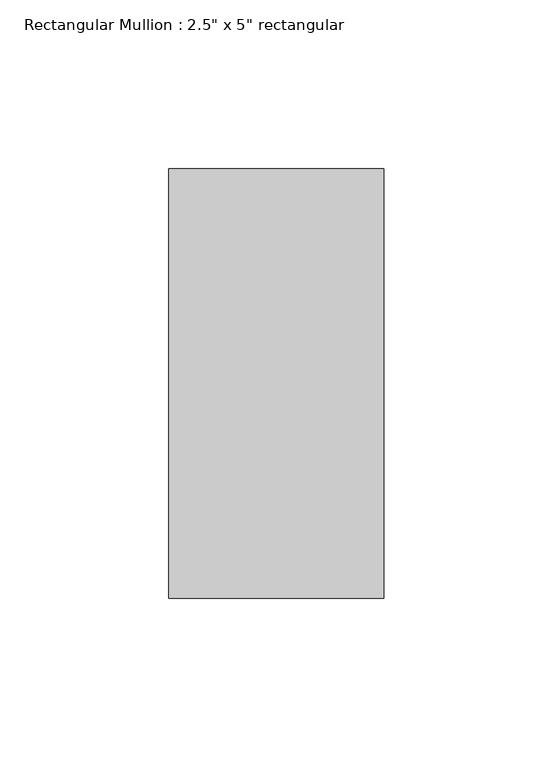
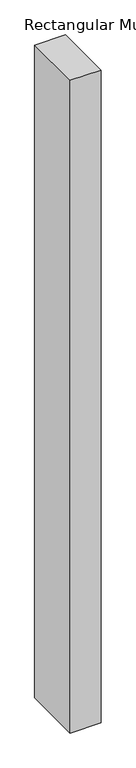
"""IFC4 building model written with IfcOpenShell, lengths in millimetres: member geometry."""

from ifc_helpers import new_model, si_unit, frame, origin, place, context, project, spatial, polyline, outline, extrude, source, transform, mapped, element, save


def member_194437a1(model_context):
    return source(origin(), model_context, "Body", "SweptSolid", [
        extrude(outline(polyline([(0.0, 63.5), (0.0, -63.5), (-63.5, -63.5), (-63.5, 63.5), (0.0, 63.5)])), frame((0.0, 0.0, -1422.4), z_axis=(0.0, 0.0, 1.0), x_axis=(1.0, 0.0, 0.0)), (0.0, 0.0, 1.0), 1422.4),
    ])


if __name__ == "__main__":
    model = new_model("IFC4")
    model_context = context("Model", 3, world=origin())
    ifc_project = project(units=[si_unit("LENGTHUNIT", "METRE", prefix="MILLI")], contexts=[model_context])
    site = spatial("IfcSite", under=ifc_project)
    building = spatial("IfcBuilding", under=site)
    placement = place(None, origin())
    member_shape = member_194437a1(model_context)
    element("IfcMember", 1, ObjectType="Rectangular Mullion : 2.5\" x 5\" rectangular", at=placement, inside=building, context=model_context, shape_type="MappedRepresentation", body=[
        mapped(member_shape, transform((0.0, 0.0, 0.0), x_axis=(1.0, 0.0, 0.0), y_axis=(0.0, 1.0, 0.0), z_axis=(0.0, 0.0, 1.0))),
    ])
    save(model, "model.ifc")

# Revit data of these elements
# Type "Rectangular Mullion : 2.5\" x 5\" rectangular"
#   built-in parameter 1007304 = 0.416667 (stored number, unit not read)
#   built-in parameter 1007301 = 0.104167 (stored number, unit not read)
#   built-in parameter 1007300 = 0.104167 (stored number, unit not read)
# Element 1 (IfcMember, "Rectangular Mullion : 2.5\" x 5\" rectangular")
#   Materials on its faces: "Aluminum"
# Materials
#   "Aluminum": class "Metal", colour RGB 247 247 247, transparency 0, Description = "Aluminum 6061", Cost = 0
